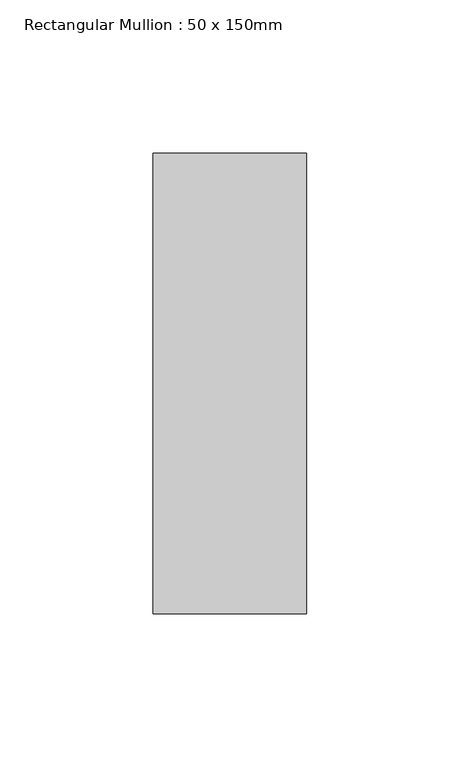
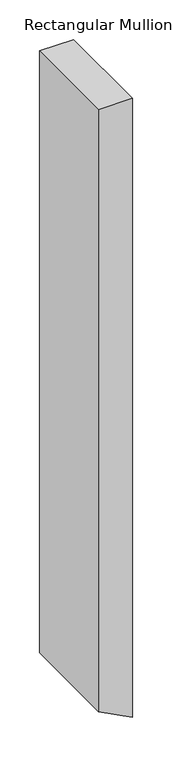
"""IFC4 building model written with IfcOpenShell, lengths in millimetres: member geometry, Rectangular Mullion : 50 x 150mm."""

from ifc_helpers import new_model, si_unit, frame, origin, place, context, project, spatial, polyline, outline, extrude, source, transform, mapped, element, save


def rectangular_mullion_50_x_150mm_cfe8f652(model_context):
    return source(origin(), model_context, "Body", "SweptSolid", [
        extrude(outline(polyline([(0.0, 0.0), (0.0, -50.0), (-929.9480713, -50.0), (-955.9764238, 0.0), (0.0, 0.0)])), frame((0.0, -75.0, 0.0), z_axis=(0.0, 1.0, 0.0), x_axis=(0.0, 0.0, 1.0)), (0.0, 0.0, 1.0), 150.0),
    ])


if __name__ == "__main__":
    model = new_model("IFC4")
    model_context = context("Model", 3, world=origin())
    ifc_project = project(units=[si_unit("LENGTHUNIT", "METRE", prefix="MILLI")], contexts=[model_context])
    site = spatial("IfcSite", under=ifc_project)
    building = spatial("IfcBuilding", under=site)
    placement = place(None, origin())
    rectangular_mullion_50_x_150mm_shape = rectangular_mullion_50_x_150mm_cfe8f652(model_context)
    element("IfcMember", 1, ObjectType="Rectangular Mullion : 50 x 150mm", at=placement, inside=building, context=model_context, shape_type="MappedRepresentation", body=[
        mapped(rectangular_mullion_50_x_150mm_shape, transform((0.0, 0.0, 0.0), x_axis=(1.0, 0.0, 0.0), y_axis=(0.0, 1.0, 0.0), z_axis=(0.0, 0.0, 1.0))),
    ])
    save(model, "model.ifc")

# Revit data of these elements
# Type "Rectangular Mullion : 50 x 150mm"
#   built-in parameter 1007304 = 0.492126 (stored number, unit not read)
#   built-in parameter 1007301 = 0.082021 (stored number, unit not read)
#   built-in parameter 1007300 = 0.082021 (stored number, unit not read)
# Element 1 (IfcMember, "Rectangular Mullion : 50 x 150mm")
#   Materials on its faces: "Aluminium"
# Materials
#   "Aluminium": class "Metal", colour RGB 247 247 247, transparency 0, Description = "Aluminium 6061", Cost = 0
